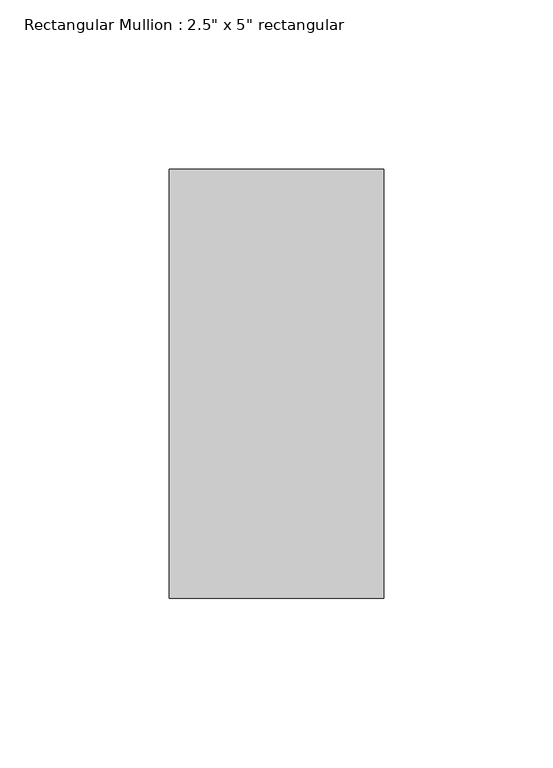
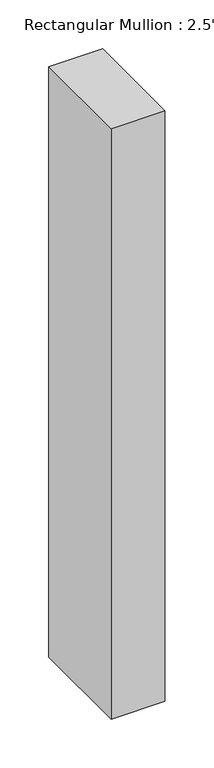
"""IFC4 building model written with IfcOpenShell, lengths in millimetres: member geometry."""

from ifc_helpers import new_model, si_unit, frame, origin, place, context, project, spatial, polyline, outline, extrude, source, transform, mapped, element, save


def member_41360271(model_context):
    return source(origin(), model_context, "Body", "SweptSolid", [
        extrude(outline(polyline([(31.75, 63.5), (31.75, -63.5), (-31.75, -63.5), (-31.75, 63.5), (31.75, 63.5)])), frame((0.0, 0.0, -736.2967564), z_axis=(0.0, 0.0, 1.0), x_axis=(1.0, 0.0, 0.0)), (0.0, 0.0, 1.0), 736.2967564),
    ])


if __name__ == "__main__":
    model = new_model("IFC4")
    model_context = context("Model", 3, world=origin())
    ifc_project = project(units=[si_unit("LENGTHUNIT", "METRE", prefix="MILLI")], contexts=[model_context])
    site = spatial("IfcSite", under=ifc_project)
    building = spatial("IfcBuilding", under=site)
    placement = place(None, origin())
    member_shape = member_41360271(model_context)
    element("IfcMember", 1, ObjectType="Rectangular Mullion : 2.5\" x 5\" rectangular", at=placement, inside=building, context=model_context, shape_type="MappedRepresentation", body=[
        mapped(member_shape, transform((0.0, 0.0, 0.0), x_axis=(1.0, 0.0, 0.0), y_axis=(0.0, 1.0, 0.0), z_axis=(0.0, 0.0, 1.0))),
    ])
    save(model, "model.ifc")

# Revit data of these elements
# Type "Rectangular Mullion : 2.5\" x 5\" rectangular"
#   built-in parameter 1007304 = 0.416667 (stored number, unit not read)
#   built-in parameter 1007301 = 0.104167 (stored number, unit not read)
#   built-in parameter 1007300 = 0.104167 (stored number, unit not read)
# Element 1 (IfcMember, "Rectangular Mullion : 2.5\" x 5\" rectangular")
#   Materials on its faces: "Aluminum"
# Materials
#   "Aluminum": class "Metal", colour RGB 247 247 247, transparency 0, Description = "Aluminum 6061", Cost = 0
